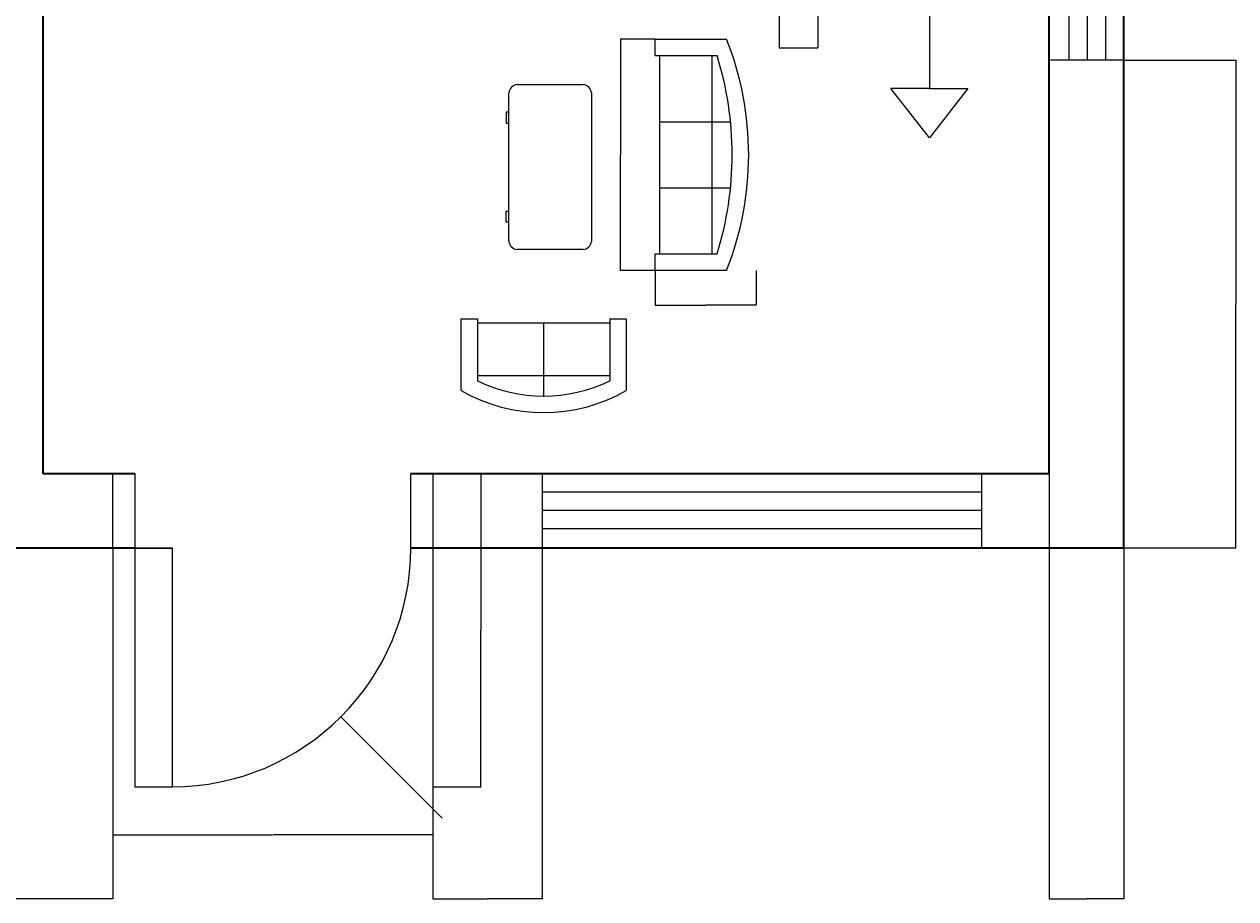
# Model space of a CAD drawing. Units: millimetres. Extents: x 726 to 37095, y -1634 to 13537.
# Tile 2 of 4: x 9102 to 17228, y -1568 to 4296. Entities that reach past the tile are written whole.
import ezdxf

# ---------------------------------------------------------------- set-up
doc = ezdxf.new("R2010")
doc.units = ezdxf.units.MM
for name, color, linetype, lineweight in [('A-ANNO-DIMS', 2, 'Continuous', 18), ('A-DOOR', 3, 'Continuous', 25), ('A-FLOR-STRS', 5, 'Continuous', 25), ('A-FURN', 8, 'Continuous', 18), ('A-GLAZ', 4, 'Continuous', 18), ('A-WALL', 7, 'Continuous', 35)]:
    doc.layers.add(name, color=color, linetype=linetype, lineweight=lineweight)
doc.styles.get("Standard").update_dxf_attribs({"font": 'arial.ttf'})
doc.dimstyles.get("Standard").update_dxf_attribs({"dimtxt": 0.18, "dimasz": 0.18, "dimexe": 0.18, "dimexo": 0.0625, "dimgap": 0.09, "dimtad": 0, "dimtih": 1, "dimtoh": 1, "dimdec": 4, "dimzin": 0, "dimdsep": 46, "dimtxsty": 'Standard', "dimcen": 0.09, "dimadec": 0, "dimazin": 0, "dimtfac": 1, "dimtdec": 4, "dimtofl": 0, "dimtmove": 0, "dimatfit": 3, "dimfxl": 1, "dimtolj": 1, "dimtzin": 0, "dimarcsym": 0})

# ---------------------------------------------------------------- blocks, each defined once
blk = doc.blocks.new('Sofa - Roundback 7 ft.')
for p, q in [((-12.00002, -32.44210000000393), (-12.00003, -6.597100000003898)), ((11.99996999999999, -32.44210000000393), (11.99997999999999, -6.597100000003898)), ((-36.000027, -34.00000000000395), (-36.000027, -11.46960000000396)), ((35.99997999999999, -34.00000000000395), (35.99997999999999, -11.46960000000396)), ((-35.999844, -13.38190000000397), (35.99979999999999, -13.38190000000397)), ((-36.000027, -32.44210000000393), (35.99997999999999, -32.44210000000393))]:
    blk.add_line(p, q)
for points in [[(-36.000027, -34.00000000000395), (-42.000027, -34.00000000000395), (-42.000027, -8.000000000003944)], [(41.99997999999999, -8.000000000003944), (41.99997999999999, -34.00000000000395), (35.99997999999999, -34.00000000000395)]]:
    blk.add_lwpolyline(points)
for centre, radius, start, end in [((0, -114.2500000000039), 114.2500000000039, 68.43141000000072, 111.5686000000006), ((-1.00000000032e-05, -127.1968000000039), 121.1967999999973, 72.72032999999948, 107.2797000000005)]:
    blk.add_arc(centre, radius, start, end)
blk = doc.blocks.new('Sofa - Roundback Loveseat 5 ft.')
for p, q in [((0, -32.44198000000246), (0, -5.999980000002448)), ((-23.99999999999999, -33.99998000000245), (-23.99999999999999, -11.46958000000243)), ((24.00004000000001, -33.99998000000245), (24.00004000000001, -11.46958000000243)), ((-23.99979999999998, -13.38178000000245), (23.99986, -13.38178000000245)), ((-23.99999999999999, -32.44198000000246), (24.00004000000001, -32.44198000000246))]:
    blk.add_line(p, q)
for points in [[(-23.99999999999999, -33.99998000000245), (-29.99999999999999, -33.99998000000245), (-29.99999999999999, -7.999980000002448)], [(30.00004000000001, -7.999980000002448), (30.00004000000001, -33.99998000000245), (24.00004000000001, -33.99998000000245)]]:
    blk.add_lwpolyline(points)
for centre, radius, start, end in [((0, -60.24998000000245), 60.24998000000245, 60.13715000000122, 119.862800000004), ((0, -61.38438000000245), 55.38444000000723, 64.32083000000306, 115.6791999999996)]:
    blk.add_arc(centre, radius, start, end)
blk = doc.blocks.new('Desk - 30 x 60 in.')
for p, q in [((-26.999995, 0), (26.999995, 0)), ((-29.999995, -27), (-29.999995, -3)), ((29.999995, -3), (29.999995, -27)), ((26.999995, -30), (-26.999995, -30)), ((-20.000005, -30), (-20.000005, -31)), ((-16.000005, -31), (-16.000005, -30)), ((15.999995, -31), (15.999995, -30)), ((19.999995, -30), (19.999995, -31)), ((-20.000005, -31), (-16.000005, -31)), ((19.999995, -31), (15.999995, -31))]:
    blk.add_line(p, q)
for centre, radius, start, end in [((-26.499995, -3.5), 3.535534000004229, 98.1300999999916, 171.8698999999352), ((26.499995, -3.5), 3.535533999997753, 8.130102000022115, 81.8698999999439), ((-26.499995, -26.5), 3.535534000000845, 188.1301000000653, 261.8699000000085), ((26.499995, -26.5), 3.535534000004826, 278.1301000000561, 351.8698999999439)]:
    blk.add_arc(centre, radius, start, end)
blk = doc.blocks.new('Window - Wood Frame 36 in. Wide plan')
for p, q in [((0, 6), (0, 0)), ((36, 6), (36, 0)), ((0, 4.5), (36, 4.5)), ((0, 3), (36, 3)), ((0, 1.5), (36, 1.5))]:
    blk.add_line(p, q)
blk = doc.blocks.new('DOOR-ENTRY-1601')
for p, q in [((0, 1600.959499914892), (0, 2101.259343638296)), ((0, 2101.259343638296), (148.488993617113, 2101.259343638296)), ((148.488993617113, 2101.259343638296), (148.488993617113, 1600.959499914892)), ((1999.598415393706, 1600.959499914892), (1999.598415393706, 2101.259343638296)), ((1999.598415393706, 2101.259343638296), (2148.087409010808, 2101.259343638296)), ((2148.087409010808, 2101.259343638296), (2148.087409010808, 1600.959499914892)), ((148.488993617113, 1600.959499914892), (0, 1600.959499914892)), ((148.488993617113, 1600.959499914892), (148.488993617113, -1.137e-13)), ((398.6389154788158, 1600.959499914892), (148.488993617113, 1600.959499914892)), ((148.488993617113, 1600.959499914892), (398.6389154788158, 1600.959499914892)), ((398.6389154788158, 1600.959499914892), (398.6389154788158, -1.137e-13)), ((2148.087409010808, 1600.959499914892), (1999.598415393706, 1600.959499914892)), ((148.488993617113, -1.137e-13), (398.6389154788158, -1.137e-13))]:
    blk.add_line(p, q)
blk.add_arc((398.6389154788158, 1600.959499914892), 1600.959499914892, 270, 0)
blk = doc.blocks.new('STAIR-QUARTER-TURN')
for p, q in [((1551.94660387568, 5000.000000000002), (1551.94660387568, 3551.516503049365)), ((1758.872817725773, 5000.000000000002), (1758.872817725773, 3551.516503049365)), ((1965.799031575862, 5000.000000000002), (1965.799031575862, 3551.516503049365)), ((2172.725245425954, 5000.000000000002), (2172.725245425954, 3551.516503049365)), ((2172.725245425954, 4193.579423830473), (803.743340616409, 4193.579423830471)), ((803.743340616409, 4193.579423830471), (803.743340616409, 330.5564002077117)), ((2172.725245425954, 3551.516503049366), (0, 3551.516503049365)), ((1551.94660387568, 3551.516503049365), (1551.94660387568, 3344.590289199272)), ((2172.725245425954, 3551.516503049365), (2172.725245425954, 3292.858735736751)), ((1551.94660387568, 3344.590289199272), (0, 3344.590289199273)), ((1551.94660387568, 3344.590289199272), (1551.94660387568, 861.4757229981805)), ((2172.725245425954, 3292.858735736751), (1810.604371188295, 3292.858735736751)), ((1810.604371188295, 3292.85873573675), (1810.604371188295, 602.8179556856148)), ((1551.94660387568, 3137.664075349182), (0, 3137.664075349182)), ((1551.94660387568, 2930.73786149909), (0, 2930.737861499091)), ((1551.94660387568, 2723.811647649), (0, 2723.811647649001)), ((1551.94660387568, 2516.885433798908), (0, 2516.885433798909)), ((1551.94660387568, 2309.959219948817), (0, 2309.959219948818)), ((1551.94660387568, 2103.033006098726), (0, 2103.033006098727)), ((1551.94660387568, 1896.106792248635), (0, 1896.106792248635)), ((1551.94660387568, 1689.180578398543), (0, 1689.180578398544)), ((1551.94660387568, 1482.254364548453), (0, 1482.254364548454)), ((1551.94660387568, 1275.328150698362), (0, 1275.328150698363)), ((1551.94660387568, 1068.40193684827), (0, 1068.401936848271)), ((1551.94660387568, 861.4757229981795), (0, 861.4757229981805)), ((1551.94660387568, 861.4757229981805), (1551.946603875687, 602.8179556856074)), ((1810.604371188295, 602.8179556856148), (1551.946603875687, 602.8179556855675)), ((803.743340616409, 330.5564002077117), (545.0855733037969, 330.5564002077117)), ((545.0855733037969, 330.5564002077117), (803.743340616409, 4.547e-13)), ((803.743340616409, 330.5564002077117), (1062.401107929021, 330.5564002077108)), ((803.743340616409, 4.547e-13), (1062.401107929021, 330.5564002077117))]:
    blk.add_line(p, q)
blk = doc.blocks.new('*D21')
at = {"layer": 'A-ANNO-DIMS', "color": 0, "lineweight": -2, "transparency": 16777216}
for p, q in [((9695.604089975648, -817.43597551541), (9695.604089975648, -1139.766586867031)), ((11843.69149898645, -817.43597551541), (11843.69149898645, -1139.766586867031)), ((9695.784089975648, -1139.586586867031), (10768.11140976072, -1139.586586867031)), ((11843.51149898645, -1139.586586867031), (10771.18417920138, -1139.586586867031))]:
    blk.add_line(p, q, dxfattribs=at)
at = {"layer": 'A-ANNO-DIMS', "color": 0, "transparency": 16777216}
for points in [[(9695.784089975648, -1139.556586867031), (9695.784089975648, -1139.616586867031), (9695.604089975648, -1139.586586867031)], [(11843.51149898645, -1139.556586867031), (11843.51149898645, -1139.616586867031), (11843.69149898645, -1139.586586867031)]]:
    blk.add_solid(points, dxfattribs=at)
at = {"layer": 'Defpoints', "color": 0, "transparency": 16777216}
for p in [(9695.604089975648, -817.3734755154098), (11843.69149898645, -817.3734755154098), (11843.69149898645, -1139.586586867031)]:
    blk.add_point(p, dxfattribs=at)
at = {"layer": 'A-ANNO-DIMS', "color": 0, "transparency": 16777216, "insert": (10769.64779448105, -1139.586586867031), "char_height": 0.18, "attachment_point": 5}
blk.add_mtext('\\A1;ENTRY DOOR 2148 TYP.', dxfattribs=at)
blk = doc.blocks.new('*D22')
at = {"layer": 'A-ANNO-DIMS', "color": 0, "lineweight": -2, "transparency": 16777216}
for p, q in [((11843.75399898646, 1283.885868122886), (12166.08461033808, 1283.885868122886)), ((12165.90461033808, 1283.705868122886), (12165.90461033808, 233.438099441528)), ((12165.90461033808, -817.1934755154103), (12165.90461033808, 233.0742931659481)), ((11843.75399898646, -817.3734755154104), (12166.08461033808, -817.3734755154102))]:
    blk.add_line(p, q, dxfattribs=at)
at = {"layer": 'A-ANNO-DIMS', "color": 0, "transparency": 16777216}
for points in [[(12165.87461033808, 1283.705868122886), (12165.93461033808, 1283.705868122886), (12165.90461033808, 1283.885868122886)], [(12165.87461033808, -817.1934755154103), (12165.93461033808, -817.1934755154103), (12165.90461033808, -817.3734755154102)]]:
    blk.add_solid(points, dxfattribs=at)
at = {"layer": 'Defpoints', "color": 0, "transparency": 16777216}
for p in [(11843.69149898646, 1283.885868122886), (12165.90461033808, 1283.885868122886), (11843.69149898646, -817.3734755154104)]:
    blk.add_point(p, dxfattribs=at)
at = {"layer": 'A-ANNO-DIMS', "color": 0, "transparency": 16777216, "insert": (12165.90461033808, 233.2561963037345), "char_height": 0.18, "attachment_point": 5}
blk.add_mtext('\\A1;2101 TYP.', dxfattribs=at)
blk = doc.blocks.new('*D25')
at = {"layer": 'A-ANNO-DIMS', "color": 0, "lineweight": -2, "transparency": 16777216}
for p, q in [((13333.54858219725, 4195.887538341497), (13100.82879643529, 4195.887538341497)), ((13101.00879643529, 4195.707538341497), (13101.00879643529, 3420.729716770213)), ((13101.00879643529, 2645.385633261685), (13101.00879643529, 3420.363454832969)), ((13333.54858219726, 2645.205633261686), (13100.82879643529, 2645.205633261685))]:
    blk.add_line(p, q, dxfattribs=at)
at = {"layer": 'A-ANNO-DIMS', "color": 0, "transparency": 16777216}
for points in [[(13100.97879643529, 4195.707538341497), (13101.03879643529, 4195.707538341497), (13101.00879643529, 4195.887538341497)], [(13100.97879643529, 2645.385633261685), (13101.03879643529, 2645.385633261685), (13101.00879643529, 2645.205633261685)]]:
    blk.add_solid(points, dxfattribs=at)
at = {"layer": 'Defpoints', "color": 0, "transparency": 16777216}
for p in [(13333.61108219725, 4195.887538341497), (13101.00879643529, 2645.205633261685), (13333.61108219726, 2645.205633261686)]:
    blk.add_point(p, dxfattribs=at)
at = {"layer": 'A-ANNO-DIMS', "color": 0, "transparency": 16777216, "insert": (13101.00879643529, 3420.546585801587), "char_height": 0.18, "attachment_point": 5}
blk.add_mtext('\\A1;SOFA 1551 TYP.', dxfattribs=at)
blk = doc.blocks.new('*D26')
at = {"layer": 'A-ANNO-DIMS', "color": 0, "lineweight": -2, "transparency": 16777216}
for p, q in [((13333.61108219725, 2645.143133261685), (13333.61108219725, 2412.423347499714)), ((14010.49592976888, 2645.143133261686), (14010.49592976888, 2412.423347499714)), ((13333.79108219725, 2412.603347499714), (13671.45499984391, 2412.603347499714)), ((14010.31592976888, 2412.603347499714), (13672.65201212222, 2412.603347499714))]:
    blk.add_line(p, q, dxfattribs=at)
at = {"layer": 'A-ANNO-DIMS', "color": 0, "transparency": 16777216}
for points in [[(13333.79108219725, 2412.633347499714), (13333.79108219725, 2412.573347499713), (13333.61108219725, 2412.603347499714)], [(14010.31592976888, 2412.633347499714), (14010.31592976888, 2412.573347499713), (14010.49592976888, 2412.603347499714)]]:
    blk.add_solid(points, dxfattribs=at)
at = {"layer": 'Defpoints', "color": 0, "transparency": 16777216}
for p in [(13333.61108219725, 2645.205633261685), (14010.49592976888, 2645.205633261686), (14010.49592976888, 2412.603347499714)]:
    blk.add_point(p, dxfattribs=at)
at = {"layer": 'A-ANNO-DIMS', "color": 0, "transparency": 16777216, "insert": (13672.05350598307, 2412.603347499714), "char_height": 0.18, "attachment_point": 5}
blk.add_mtext('\\A1;677 TYP.', dxfattribs=at)
blk = doc.blocks.new('*D52')
at = {"layer": 'A-ANNO-DIMS', "color": 0, "lineweight": -2, "transparency": 16777216}
for p, q in [((15977.309846, 1283.823368), (15977.309846, -1568.303476)), ((16477.309846, 783.823368), (16477.309846, -1568.303476)), ((15977.489846, -1568.123476), (16227.02130575443, -1568.123476)), ((16477.129846, -1568.123476), (16227.59838624556, -1568.123476))]:
    blk.add_line(p, q, dxfattribs=at)
at = {"layer": 'A-ANNO-DIMS', "color": 0, "transparency": 16777216}
for points in [[(15977.489846, -1568.093476), (15977.489846, -1568.153476), (15977.309846, -1568.123476)], [(16477.129846, -1568.093476), (16477.129846, -1568.153476), (16477.309846, -1568.123476)]]:
    blk.add_solid(points, dxfattribs=at)
at = {"layer": 'Defpoints', "color": 0, "transparency": 16777216}
for p in [(15977.309846, 1283.885868), (16477.309846, 783.8858679999998), (16477.309846, -1568.123476)]:
    blk.add_point(p, dxfattribs=at)
at = {"layer": 'A-ANNO-DIMS', "color": 0, "transparency": 16777216, "insert": (16227.309846, -1568.123476), "char_height": 0.18, "attachment_point": 5}
blk.add_mtext('\\A1;500', dxfattribs=at)
blk = doc.blocks.new('*D59')
at = {"layer": 'A-ANNO-DIMS', "color": 0, "lineweight": -2, "transparency": 16777216}
for p, q in [((8127.064238, 783.523524), (8127.064238, -1568.303476)), ((9695.60409, 783.523524), (9695.60409, -1568.303476)), ((8127.244238000001, -1568.123476), (8910.878331803548, -1568.123476)), ((9695.42409, -1568.123476), (8911.789996196452, -1568.123476))]:
    blk.add_line(p, q, dxfattribs=at)
at = {"layer": 'A-ANNO-DIMS', "color": 0, "transparency": 16777216}
for points in [[(8127.244238000001, -1568.093476), (8127.244238000001, -1568.153476), (8127.064238, -1568.123476)], [(9695.42409, -1568.093476), (9695.42409, -1568.153476), (9695.60409, -1568.123476)]]:
    blk.add_solid(points, dxfattribs=at)
at = {"layer": 'Defpoints', "color": 0, "transparency": 16777216}
for p in [(8127.064238, 783.586024), (9695.60409, 783.586024), (9695.60409, -1568.123476)]:
    blk.add_point(p, dxfattribs=at)
at = {"layer": 'A-ANNO-DIMS', "color": 0, "transparency": 16777216, "insert": (8911.334164000002, -1568.123476), "char_height": 0.18, "attachment_point": 5}
blk.add_mtext('\\A1;1568.5', dxfattribs=at)
blk = doc.blocks.new('*D60')
at = {"layer": 'A-ANNO-DIMS', "color": 0, "lineweight": -2, "transparency": 16777216}
for p, q in [((11843.691499, 783.523524), (11843.691499, -1568.303476)), ((12575.488099, 792.4362369999999), (12575.488099, -1568.303476)), ((11843.871499, -1568.123476), (12209.19664756753, -1568.123476)), ((12575.308099, -1568.123476), (12209.98295043247, -1568.123476))]:
    blk.add_line(p, q, dxfattribs=at)
at = {"layer": 'A-ANNO-DIMS', "color": 0, "transparency": 16777216}
for points in [[(11843.871499, -1568.093476), (11843.871499, -1568.153476), (11843.691499, -1568.123476)], [(12575.308099, -1568.093476), (12575.308099, -1568.153476), (12575.488099, -1568.123476)]]:
    blk.add_solid(points, dxfattribs=at)
at = {"layer": 'Defpoints', "color": 0, "transparency": 16777216}
for p in [(11843.691499, 783.586024), (12575.488099, 792.498737), (12575.488099, -1568.123476)]:
    blk.add_point(p, dxfattribs=at)
at = {"layer": 'A-ANNO-DIMS', "color": 0, "transparency": 16777216, "insert": (12209.589799, -1568.123476), "char_height": 0.18, "attachment_point": 5}
blk.add_mtext('\\A1;731.8', dxfattribs=at)
blk = doc.blocks.new('*D61')
at = {"layer": 'A-ANNO-DIMS', "color": 0, "lineweight": -2, "transparency": 16777216}
for p, q in [((16477.372346, 4054.816655000002), (17228.23984600001, 4054.816655000002)), ((17228.05984600001, 4054.636655000002), (17228.05984600001, 2419.533226029333)), ((17228.05984600001, 784.0658680000005), (17228.05984600001, 2419.16929697067)), ((16477.372346, 783.8858680000003), (17228.23984600001, 783.8858680000006))]:
    blk.add_line(p, q, dxfattribs=at)
at = {"layer": 'A-ANNO-DIMS', "color": 0, "transparency": 16777216}
for points in [[(17228.02984600001, 4054.636655000002), (17228.08984600001, 4054.636655000002), (17228.05984600001, 4054.816655000002)], [(17228.02984600001, 784.0658680000005), (17228.08984600001, 784.0658680000005), (17228.05984600001, 783.8858680000006)]]:
    blk.add_solid(points, dxfattribs=at)
at = {"layer": 'Defpoints', "color": 0, "transparency": 16777216}
for p in [(16477.309846, 4054.816655000002), (17228.05984600001, 4054.816655000002), (16477.309846, 783.8858680000003)]:
    blk.add_point(p, dxfattribs=at)
at = {"layer": 'A-ANNO-DIMS', "color": 0, "transparency": 16777216, "insert": (17228.05984600001, 2419.351261499997), "char_height": 0.18, "attachment_point": 5}
blk.add_mtext('\\A1;3271', dxfattribs=at)
blk = doc.blocks.new('*D86')
at = {"layer": 'A-ANNO-DIMS', "color": 0, "lineweight": -2, "transparency": 16777216}
for p, q in [((10094.153005, 783.5860240000002), (10094.333005, 783.5860240000002)), ((10094.243005, 783.496024), (10094.243005, 783.6760240000003)), ((11905.52189161301, -1027.692909013012), (11226.41958821898, -348.5905882222433)), ((11905.70189161301, -1027.692909013012), (11905.52189161301, -1027.692909013012))]:
    blk.add_line(p, q, dxfattribs=at)
at = {"layer": 'A-ANNO-DIMS', "color": 0, "transparency": 16777216}
blk.add_solid([(11226.44080142269, -348.5693750190794), (11226.39837501527, -348.6118014254071), (11226.292309, -348.4633089999998)], dxfattribs=at)
at = {"layer": 'Defpoints', "color": 0, "transparency": 16777216}
for p in [(10094.243005, 783.5860240000002), (11226.292309, -348.4633089999998)]:
    blk.add_point(p, dxfattribs=at)
at = {"layer": 'A-ANNO-DIMS', "color": 0, "transparency": 16777216, "insert": (11906.32434045339, -1027.692909013011), "char_height": 0.18, "attachment_point": 5}
blk.add_mtext('\\A1;2X R1601', dxfattribs=at)

msp = doc.modelspace()

# ---------------------------------------------------------------- linework, layer by layer
at = {"layer": 'A-WALL'}
for p, q in [((16477.30984586529, 783.8858681228857), (16477.30984586529, 12783.88586812288)), ((9227.30984586529, 8533.885868122885), (9227.30984586529, 1283.885868122886)), ((15977.30984586529, 1283.885868122886), (15977.30984586529, 8533.885868122885)), ((9227.30984586529, 1283.885868122886), (9844.093083592761, 1283.885868122885)), ((11695.20250536935, 1283.885868122885), (15977.30984586529, 1283.885868122886)), ((7978.5752445832, 783.8858681228859), (9844.093083592761, 783.8858681228859)), ((11695.20250536935, 783.8858681228859), (16477.30984586529, 783.8858681228857))]:
    msp.add_line(p, q, dxfattribs=at)

# ---------------------------------------------------------------- block references
at = {"layer": 'A-DOOR'}
msp.add_blockref('DOOR-ENTRY-1601', (9695.604089975648, -817.3734755154098), dxfattribs=at)
at = {"layer": 'A-FLOR-STRS', "extrusion": (0, 0, -1), "zscale": -1}
msp.add_blockref('STAIR-QUARTER-TURN', (-15977.30984586528, 3533.885868122882), dxfattribs=at)
at = {"layer": 'A-FURN', "xscale": 18.46049527356076, "yscale": 18.46049527356076, "zscale": 18.46049527356076}
for name, p, rotation in [('Sofa - Roundback 7 ft.', (13961.26792149839, 3420.546238418572), 270.0000000000001), ('Desk - 30 x 60 in.', (12906.55733993705, 3337.924817260524), 270.0000000000001), ('Sofa - Roundback Loveseat 5 ft.', (12585.96045986141, 1691.694815374398), 180)]:
    msp.add_blockref(name, p, dxfattribs=dict(at, rotation=rotation))
at = {"layer": 'A-GLAZ', "xscale": 81.8978551733564, "yscale": 81.8978551733564, "zscale": 81.8978551733564, "rotation": 270}
msp.add_blockref('Window - Wood Frame 36 in. Wide plan', (15985.92271482514, 7003.139441062607), dxfattribs=at)
at = {"layer": 'A-GLAZ', "xscale": 81.8978551733564, "yscale": 81.8978551733564, "zscale": 81.8978551733564}
msp.add_blockref('Window - Wood Frame 36 in. Wide plan', (12575.48809910245, 792.4987370827457), dxfattribs=at)

# ---------------------------------------------------------------- dimensions: what is measured, and where the dimension line sits
at = {"layer": 'A-ANNO-DIMS'}
for base, p1, p2, angle, text, picture, middle in [((13101.00879643529, 2645.205633261685), (13333.61108219725, 4195.887538341495), (13333.61108219725, 2645.205633261685), 270.0000000000001, 'SOFA <> TYP.', '*D25', (13101.00879643529, 3420.546585801587)), ((14010.49592976888, 2412.603347499714), (13333.61108219725, 2645.205633261685), (14010.49592976888, 2645.205633261686), 1.155e-13, '<> TYP.', '*D26', (13672.05350598307, 2412.603347499714)), ((12165.90461033808, 1283.885868122886), (11843.69149898645, -817.3734755154098), (11843.69149898645, 1283.885868122886), 90, '<> TYP.', '*D22', (12165.90461033808, 233.2561963037345))]:
    dim = msp.add_linear_dim(base=base, p1=p1, p2=p2, angle=angle, text=text, dimstyle='Standard', override={"dimdec": 0, "dimlfac": 1, "dimrnd": 0, "dimzin": 0, "dimdsep": 46, "dimlunit": 2}, dxfattribs=at)
    dim.commit()
    dim.dimension.update_dxf_attribs({"geometry": picture, "text_midpoint": middle})
dim = msp.add_linear_dim(base=(17228.05984600001, 4054.816655000002), p1=(16477.309846, 783.8858679999998), p2=(16477.309846, 4054.816655), angle=90, dimstyle='Standard', override={"dimdec": 0, "dimlfac": 1, "dimrnd": 0, "dimzin": 0, "dimdsep": 46, "dimlunit": 2}, dxfattribs=at)
dim.commit()
dim.dimension.update_dxf_attribs({"geometry": '*D61', "text_midpoint": (17228.05984600001, 2419.351261499997)})
for base, p1, p2, override, picture, middle in [((16477.309846, -1568.123476), (15977.309846, 1283.885868), (16477.309846, 783.8858679999998), {"dimdec": 0, "dimlfac": 1, "dimrnd": 0, "dimzin": 0, "dimdsep": 46, "dimlunit": 2}, '*D52', (16227.309846, -1568.123476)), ((9695.60409, -1568.123476), (8127.064238, 783.586024), (9695.60409, 783.586024), {"dimdec": 1, "dimlfac": 1, "dimrnd": 0, "dimzin": 0, "dimdsep": 46, "dimlunit": 2}, '*D59', (8911.334164000002, -1568.123476)), ((12575.488099, -1568.123476), (11843.691499, 783.586024), (12575.488099, 792.498737), {"dimdec": 1, "dimlfac": 1, "dimrnd": 0, "dimzin": 0, "dimdsep": 46, "dimlunit": 2}, '*D60', (12209.589799, -1568.123476))]:
    dim = msp.add_linear_dim(base=base, p1=p1, p2=p2, dimstyle='Standard', override=override, dxfattribs=at)
    dim.commit()
    dim.dimension.update_dxf_attribs({"geometry": picture, "text_midpoint": middle})
dim = msp.add_radius_dim(center=(10094.243005, 783.5860240000002), mpoint=(11226.292309, -348.4633089999998), text='2X <>', dimstyle='Standard', override={"dimdec": 0, "dimlfac": 1, "dimrnd": 0, "dimzin": 0, "dimdsep": 46, "dimlunit": 2}, dxfattribs=at)
dim.commit()
dim.dimension.update_dxf_attribs({"geometry": '*D86', "text_midpoint": (11906.32434045339, -1027.692909013011), "dimtype": 164})
dim = msp.add_linear_dim(base=(11843.69149898645, -1139.586586867031), p1=(9695.604089975648, -817.3734755154098), p2=(11843.69149898645, -817.3734755154098), text='ENTRY DOOR <> TYP.', dimstyle='Standard', override={"dimdec": 0, "dimlfac": 1, "dimrnd": 0, "dimzin": 0, "dimdsep": 46, "dimlunit": 2}, dxfattribs=at)
dim.commit()
dim.dimension.update_dxf_attribs({"geometry": '*D21', "text_midpoint": (10769.64779448105, -1139.586586867031)})

doc.saveas('drawing.dxf')
